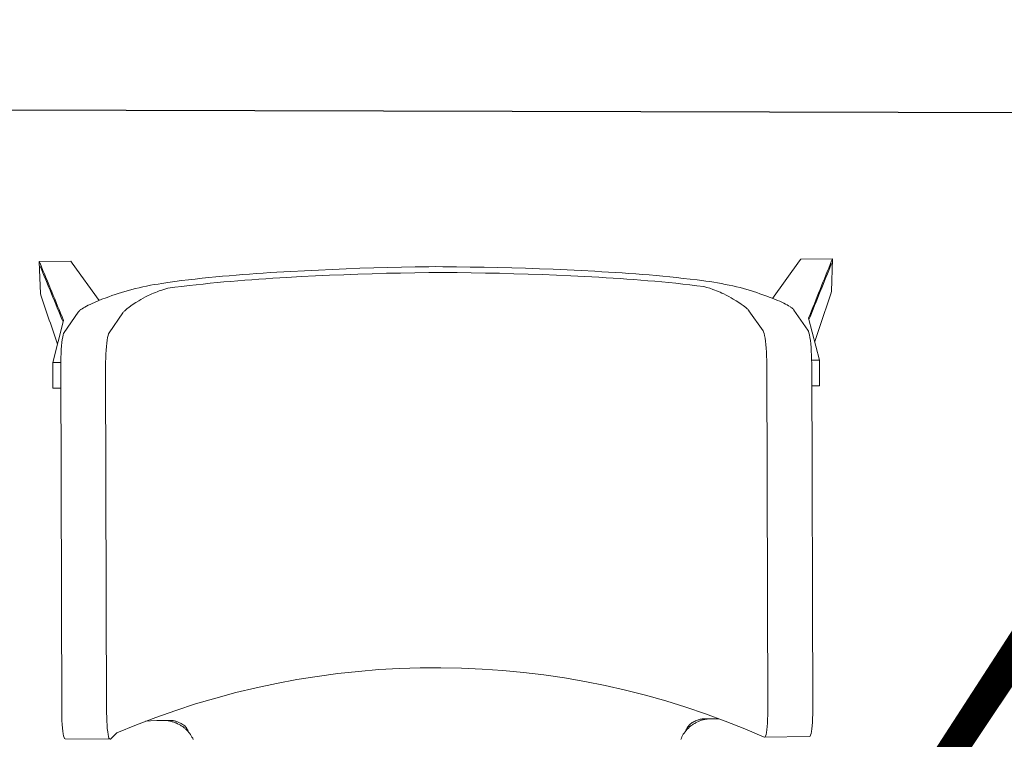
# Model space of a CAD drawing. Units: inches. Extents: x -466983 to 1020, y 324 to 318697.
# Tile 36 of 97: x 867.6 to 887.72, y 741.96 to 756.67. Entities that reach past the tile are written whole.
import ezdxf

# ---------------------------------------------------------------- set-up
doc = ezdxf.new("R2010")
doc.units = ezdxf.units.IN
doc.header["$MEASUREMENT"] = 0
for name, color, linetype, lineweight in [('A-ANNO-DIMS', 2, 'Continuous', 18), ('A-FLOR-PATT', 252, 'Continuous', 13), ('A-FURN', 8, 'Continuous', 18)]:
    doc.layers.add(name, color=color, linetype=linetype, lineweight=lineweight)
doc.layers.add('Office Desk', color=30, linetype='Continuous', true_color=0xeb7500)
doc.styles.get("Standard").update_dxf_attribs({"font": 'arial.ttf'})
doc.dimstyles.get("Standard").update_dxf_attribs({"dimtxt": 6, "dimasz": 4, "dimexe": 3, "dimexo": 3, "dimgap": 0.09, "dimtad": 0, "dimtih": 1, "dimtoh": 1, "dimdec": 1, "dimzin": 0, "dimdsep": 46, "dimlunit": 3, "dimtxsty": 'Standard', "dimcen": 0.09, "dimadec": 0, "dimazin": 0, "dimtfac": 1, "dimtdec": 1, "dimtofl": 0, "dimtmove": 0, "dimatfit": 3, "dimfxl": 1, "dimtolj": 1, "dimtzin": 0, "dimarcsym": 0})

# ---------------------------------------------------------------- blocks, each defined once
blk = doc.blocks.new('Offce Table')
at = {"layer": 'Office Desk'}
blk.add_line((2575.658, 950.355, -0.016), (2635.658, 950.194, -0.016), dxfattribs=at)
blk = doc.blocks.new('Office Chairs')
at = {"ltscale": 60}
for p, q in [((4347, 1436), (4348.4, 1437.9)), ((4382.1, 1438), (4348.4, 1437.9)), ((4382.1, 1438), (4381.1, 1403.3)), ((4382.1, 1438), (4381.3, 1436)), ((3537.6, 1435.4), (3571.3, 1435.6)), ((3537.6, 1435.4), (3538.4, 1433.4)), ((3537.6, 1435.4), (3538.8, 1400.8)), ((3572.7, 1433.6), (3571.3, 1435.6)), ((3601.5, 1393.8), (3572.7, 1433.6)), ((3820.1, 1425.5), (3834.9, 1426.2)), ((3834.9, 1426.2), (3849.6, 1426.9)), ((3849.6, 1426.9), (3864.3, 1427.5)), ((3864.3, 1427.5), (3879.1, 1428)), ((3879.1, 1428), (3893.8, 1428.4)), ((3893.8, 1428.4), (3908.6, 1428.8)), ((3908.6, 1428.8), (3923.3, 1429.2)), ((3923.3, 1429.2), (3937.9, 1429.5)), ((3937.9, 1429.5), (3952.6, 1429.7)), ((3952.6, 1429.7), (3959.9, 1429.8)), ((3967.2, 1429.7), (3959.9, 1429.8)), ((3981.9, 1429.6), (3967.2, 1429.7)), ((3996.5, 1429.4), (3981.9, 1429.6)), ((4011.3, 1429.2), (3996.5, 1429.4)), ((4026, 1428.8), (4011.3, 1429.2)), ((4040.8, 1428.5), (4026, 1428.8)), ((4055.5, 1428), (4040.8, 1428.5)), ((4070.3, 1427.5), (4055.5, 1428)), ((4085, 1427), (4070.3, 1427.5)), ((4099.8, 1426.3), (4085, 1427)), ((4114.5, 1425.6), (4099.8, 1426.3)), ((4318.5, 1396), (4347, 1436)), ((3689.2, 1414.9), (3696.5, 1415.7)), ((3696.5, 1415.7), (3703.8, 1416.6)), ((3703.8, 1416.6), (3711.1, 1417.4)), ((3711.1, 1417.4), (3718.3, 1418.1)), ((3718.3, 1418.1), (3725.5, 1418.8)), ((3725.5, 1418.8), (3732.8, 1419.5)), ((3732.8, 1419.5), (3740, 1420.1)), ((3740, 1420.1), (3747.2, 1420.7)), ((3747.2, 1420.7), (3754.4, 1421.3)), ((3749.1, 1414.7), (3756.5, 1415.3)), ((3754.4, 1421.3), (3761.6, 1421.9)), ((3756.5, 1415.3), (3763.9, 1415.9)), ((3761.6, 1421.9), (3768.9, 1422.4)), ((3763.9, 1415.9), (3771.4, 1416.4)), ((3768.9, 1422.4), (3776.1, 1422.9)), ((3771.4, 1416.4), (3778.8, 1416.9)), ((3776.1, 1422.9), (3783.4, 1423.4)), ((3778.8, 1416.9), (3786.3, 1417.4)), ((3783.4, 1423.4), (3790.7, 1423.8)), ((3786.3, 1417.4), (3793.8, 1417.9)), ((3790.7, 1423.8), (3805.4, 1424.7)), ((3793.8, 1417.9), (3801.3, 1418.3)), ((3801.3, 1418.3), (3816.4, 1419.2)), ((3805.4, 1424.7), (3820.1, 1425.5)), ((3816.4, 1419.2), (3831.6, 1419.9)), ((3831.6, 1419.9), (3846.7, 1420.6)), ((3846.7, 1420.6), (3861.8, 1421.2)), ((3861.8, 1421.2), (3877, 1421.8)), ((3877, 1421.8), (3892.1, 1422.3)), ((3892.1, 1422.3), (3907.2, 1422.7)), ((3907.2, 1422.7), (3922.4, 1423)), ((3922.4, 1423), (3937.4, 1423.3)), ((3937.4, 1423.3), (3952.4, 1423.6)), ((3952.4, 1423.6), (3959.9, 1423.6)), ((3967.5, 1423.6), (3959.9, 1423.6)), ((3982.5, 1423.5), (3967.5, 1423.6)), ((3997.5, 1423.3), (3982.5, 1423.5)), ((4012.7, 1423), (3997.5, 1423.3)), ((4027.8, 1422.7), (4012.7, 1423)), ((4042.9, 1422.3), (4027.8, 1422.7)), ((4058.1, 1421.8), (4042.9, 1422.3)), ((4073.2, 1421.3), (4058.1, 1421.8)), ((4088.3, 1420.7), (4073.2, 1421.3)), ((4103.5, 1420), (4088.3, 1420.7)), ((4118.6, 1419.3), (4103.5, 1420)), ((4129.2, 1424.9), (4114.5, 1425.6)), ((4126.1, 1418.9), (4118.6, 1419.3)), ((4133.6, 1418.5), (4126.1, 1418.9)), ((4136.5, 1424.4), (4129.2, 1424.9)), ((4141.1, 1418), (4133.6, 1418.5)), ((4143.8, 1424), (4136.5, 1424.4)), ((4148.6, 1417.6), (4141.1, 1418)), ((4151, 1423.5), (4143.8, 1424)), ((4156, 1417.1), (4148.6, 1417.6)), ((4158.3, 1423.1), (4151, 1423.5)), ((4163.4, 1416.6), (4156, 1417.1)), ((4165.5, 1422.6), (4158.3, 1423.1)), ((4170.8, 1416), (4163.4, 1416.6)), ((4172.7, 1422), (4165.5, 1422.6)), ((4178.2, 1415.4), (4170.8, 1416)), ((4179.9, 1421.5), (4172.7, 1422)), ((4185.6, 1414.8), (4178.2, 1415.4)), ((4187.1, 1420.9), (4179.9, 1421.5)), ((4194.4, 1420.2), (4187.1, 1420.9)), ((4201.6, 1419.6), (4194.4, 1420.2)), ((4208.9, 1418.9), (4201.6, 1419.6)), ((4216.1, 1418.1), (4208.9, 1418.9)), ((4223.4, 1417.3), (4216.1, 1418.1)), ((4230.7, 1416.5), (4223.4, 1417.3)), ((4238.1, 1415.6), (4230.7, 1416.5)), ((4245.4, 1414.7), (4238.1, 1415.6)), ((3632.5, 1404.4), (3636.2, 1405.4)), ((3636.2, 1405.4), (3640, 1406.4)), ((3640, 1406.4), (3643.9, 1407.3)), ((3643.9, 1407.3), (3647.9, 1408.2)), ((3647.9, 1408.2), (3651.9, 1409)), ((3651.9, 1409), (3656, 1409.9)), ((3656, 1409.9), (3660, 1410.6)), ((3660, 1410.6), (3664.2, 1411.3)), ((3664.2, 1411.3), (3668.3, 1412)), ((3665.3, 1403.9), (3668.3, 1404.9)), ((3668.3, 1412), (3672.5, 1412.6)), ((3668.3, 1404.9), (3671.4, 1405.9)), ((3671.4, 1405.9), (3674.6, 1406.8)), ((3672.5, 1412.6), (3674.5, 1412.9)), ((3674.5, 1412.9), (3681.9, 1413.9)), ((3674.6, 1406.8), (3682.1, 1407.8)), ((3681.9, 1413.9), (3689.2, 1414.9)), ((3682.1, 1407.8), (3689.6, 1408.8)), ((3689.6, 1408.8), (3697.1, 1409.7)), ((3697.1, 1409.7), (3704.6, 1410.5)), ((3704.6, 1410.5), (3712, 1411.3)), ((3712, 1411.3), (3719.5, 1412.1)), ((3719.5, 1412.1), (3726.9, 1412.8)), ((3726.9, 1412.8), (3734.3, 1413.5)), ((3734.3, 1413.5), (3741.7, 1414.1)), ((3741.7, 1414.1), (3749.1, 1414.7)), ((4193.1, 1414.2), (4185.6, 1414.8)), ((4200.5, 1413.5), (4193.1, 1414.2)), ((4207.9, 1412.8), (4200.5, 1413.5)), ((4215.4, 1412.1), (4207.9, 1412.8)), ((4222.9, 1411.3), (4215.4, 1412.1)), ((4230.4, 1410.4), (4222.9, 1411.3)), ((4237.9, 1409.5), (4230.4, 1410.4)), ((4245.4, 1408.5), (4237.9, 1409.5)), ((4247.5, 1414.4), (4245.4, 1414.7)), ((4248.6, 1407.6), (4245.4, 1408.5)), ((4251.6, 1413.8), (4247.5, 1414.4)), ((4251.7, 1406.7), (4248.6, 1407.6)), ((4255.8, 1413.1), (4251.6, 1413.8)), ((4254.7, 1405.6), (4251.7, 1406.7)), ((4256.8, 1404.9), (4254.7, 1405.6)), ((4259.9, 1412.4), (4255.8, 1413.1)), ((4258.8, 1404.2), (4256.8, 1404.9)), ((4264, 1411.7), (4259.9, 1412.4)), ((4268.1, 1410.9), (4264, 1411.7)), ((4272.1, 1410.1), (4268.1, 1410.9)), ((4276, 1409.2), (4272.1, 1410.1)), ((4279.9, 1408.3), (4276, 1409.2)), ((4283.8, 1407.4), (4279.9, 1408.3)), ((4287.5, 1406.4), (4283.8, 1407.4)), ((4291.2, 1405.4), (4287.5, 1406.4)), ((4294.8, 1404.3), (4291.2, 1405.4)), ((3539.6, 1398.4), (3538.8, 1400.8)), ((3600.3, 1393.3), (3604.4, 1395)), ((3604.4, 1395), (3608.8, 1396.7)), ((3608.8, 1396.7), (3611.8, 1397.8)), ((3611.8, 1397.8), (3615, 1398.9)), ((3615, 1398.9), (3618.3, 1400.1)), ((3618.3, 1400.1), (3621.7, 1401.2)), ((3621.7, 1401.2), (3625.2, 1402.3)), ((3625.2, 1402.3), (3628.8, 1403.4)), ((3628.8, 1403.4), (3632.5, 1404.4)), ((3643.5, 1393.4), (3645.9, 1394.8)), ((3645.9, 1394.8), (3648.4, 1396.2)), ((3648.4, 1396.2), (3650.9, 1397.6)), ((3650.9, 1397.6), (3653.6, 1399)), ((3653.6, 1399), (3655.5, 1399.9)), ((3655.5, 1399.9), (3657.4, 1400.7)), ((3657.4, 1400.7), (3659.3, 1401.5)), ((3659.3, 1401.5), (3661.3, 1402.3)), ((3661.3, 1402.3), (3663.2, 1403.1)), ((3663.2, 1403.1), (3665.3, 1403.9)), ((4260.7, 1403.4), (4258.8, 1404.2)), ((4262.7, 1402.6), (4260.7, 1403.4)), ((4264.5, 1401.7), (4262.7, 1402.6)), ((4266.4, 1400.9), (4264.5, 1401.7)), ((4269.1, 1399.5), (4266.4, 1400.9)), ((4271.7, 1398.1), (4269.1, 1399.5)), ((4274.2, 1396.7), (4271.7, 1398.1)), ((4276.6, 1395.3), (4274.2, 1396.7)), ((4279.6, 1393.5), (4276.6, 1395.3)), ((4298.3, 1403.2), (4294.8, 1404.3)), ((4301.7, 1402.1), (4298.3, 1403.2)), ((4305, 1401), (4301.7, 1402.1)), ((4308.2, 1399.9), (4305, 1401)), ((4311.3, 1398.8), (4308.2, 1399.9)), ((4315.7, 1397.1), (4311.3, 1398.8)), ((4319.8, 1395.5), (4315.7, 1397.1)), ((4323.6, 1393.9), (4319.8, 1395.5)), ((4380.3, 1401), (4381.1, 1403.3)), ((3581.4, 1383.7), (3581.9, 1384.1)), ((3581.9, 1384.1), (3582.5, 1384.5)), ((3582.5, 1384.5), (3583.2, 1385)), ((3583.2, 1385), (3584.6, 1385.9)), ((3584.6, 1385.9), (3586.2, 1386.8)), ((3586.2, 1386.8), (3587.9, 1387.7)), ((3587.9, 1387.7), (3589.8, 1388.7)), ((3589.8, 1388.7), (3591.9, 1389.6)), ((3591.9, 1389.6), (3594.1, 1390.7)), ((3594.1, 1390.7), (3596.4, 1391.7)), ((3596.4, 1391.7), (3600.3, 1393.3)), ((3629.4, 1383.6), (3630.1, 1384.2)), ((3630.1, 1384.2), (3631.4, 1385.3)), ((3631.4, 1385.3), (3632.9, 1386.4)), ((3632.9, 1386.4), (3635.2, 1388)), ((3635.2, 1388), (3637.7, 1389.7)), ((3637.7, 1389.7), (3640.5, 1391.5)), ((3640.5, 1391.5), (3643.5, 1393.4)), ((4282.4, 1391.7), (4279.6, 1393.5)), ((4284.9, 1390), (4282.4, 1391.7)), ((4287.2, 1388.4), (4284.9, 1390)), ((4288.7, 1387.3), (4287.2, 1388.4)), ((4290, 1386.2), (4288.7, 1387.3)), ((4290.8, 1385.6), (4290, 1386.2)), ((4291.5, 1385), (4290.8, 1385.6)), ((4292.1, 1384.4), (4291.5, 1385)), ((4292.6, 1383.8), (4292.1, 1384.4)), ((4326, 1392.9), (4323.6, 1393.9)), ((4328.2, 1391.9), (4326, 1392.9)), ((4330.3, 1390.9), (4328.2, 1391.9)), ((4332.2, 1390), (4330.3, 1390.9)), ((4333.9, 1389), (4332.2, 1390)), ((4335.5, 1388.1), (4333.9, 1389)), ((4337, 1387.3), (4335.5, 1388.1)), ((4337.6, 1386.8), (4337, 1387.3)), ((4338.2, 1386.4), (4337.6, 1386.8)), ((4338.8, 1386), (4338.2, 1386.4)), ((4339.3, 1385.6), (4338.8, 1386)), ((4339.7, 1385.2), (4339.3, 1385.6)), ((4340.2, 1384.8), (4339.7, 1385.2)), ((4340.5, 1384.4), (4340.2, 1384.8)), ((4340.9, 1384), (4340.5, 1384.4)), ((4341.2, 1383.6), (4340.9, 1384)), ((3564.2, 1359.8), (3579, 1381.3)), ((3579, 1381.3), (3579.3, 1381.7)), ((3579.3, 1381.7), (3579.6, 1382.1)), ((3579.6, 1382.1), (3580, 1382.5)), ((3580, 1382.5), (3580.4, 1382.9)), ((3580.4, 1382.9), (3580.9, 1383.3)), ((3580.9, 1383.3), (3581.4, 1383.7)), ((3612, 1359.2), (3626.8, 1380.7)), ((3626.8, 1380.7), (3627.1, 1381.2)), ((3627.1, 1381.2), (3627.6, 1381.8)), ((3627.6, 1381.8), (3628.1, 1382.3)), ((3628.1, 1382.3), (3628.7, 1382.9)), ((3628.7, 1382.9), (3629.4, 1383.6)), ((4293, 1383.2), (4292.6, 1383.8)), ((4293.3, 1382.7), (4293, 1383.2)), ((4308.3, 1361.3), (4293.3, 1382.7)), ((4356.1, 1362.2), (4341.2, 1383.6)), ((4368.5, 1330.2), (4356.7, 1375)), ((3552, 1327.7), (3563.5, 1372.6)), ((3562.1, 1352.1), (3562.6, 1354.8)), ((3562.6, 1354.8), (3563.1, 1357)), ((3563.1, 1357), (3563.6, 1358.7)), ((3563.6, 1358.7), (3564.2, 1359.8)), ((3610, 1351.4), (3610.4, 1354.2)), ((3610.4, 1354.2), (3610.9, 1356.4)), ((3610.9, 1356.4), (3611.5, 1358.1)), ((3611.5, 1358.1), (3612, 1359.2)), ((4308.3, 1361.3), (4308.9, 1360.2)), ((4308.9, 1360.2), (4309.4, 1358.5)), ((4309.4, 1358.5), (4309.9, 1356.3)), ((4309.9, 1356.3), (4310.4, 1353.6)), ((4310.4, 1353.6), (4310.9, 1350.4)), ((4356.1, 1362.2), (4356.7, 1361.1)), ((4356.7, 1361.1), (4357.2, 1359.4)), ((4357.2, 1359.4), (4357.8, 1357.2)), ((4357.8, 1357.2), (4358.2, 1354.5)), ((4358.2, 1354.5), (4358.7, 1351.3)), ((3561, 1341.4), (3561.3, 1345.3)), ((3561.3, 1345.3), (3561.7, 1348.9)), ((3561.7, 1348.9), (3562.1, 1352.1)), ((3608.8, 1340.8), (3609.2, 1344.7)), ((3609.2, 1344.7), (3609.5, 1348.3)), ((3609.5, 1348.3), (3610, 1351.4)), ((4310.9, 1350.4), (4311.2, 1346.8)), ((4311.2, 1346.8), (4311.6, 1342.9)), ((4311.6, 1342.9), (4311.9, 1338.8)), ((4358.7, 1351.3), (4359.1, 1347.7)), ((4359.1, 1347.7), (4359.4, 1343.8)), ((4359.4, 1343.8), (4359.7, 1339.7)), ((3560.5, 1328.5), (3560.6, 1333)), ((3560.6, 1333), (3560.8, 1337.3)), ((3560.8, 1337.3), (3561, 1341.4)), ((3608.3, 1327.9), (3608.4, 1332.3)), ((3608.4, 1332.3), (3608.6, 1336.6)), ((3608.6, 1336.6), (3608.8, 1340.8)), ((4311.9, 1338.8), (4312.1, 1334.5)), ((4312.1, 1334.5), (4312.2, 1330.1)), ((4359.7, 1339.7), (4359.9, 1335.4)), ((4359.9, 1335.4), (4360, 1331)), ((3552, 1327.7), (3555.2, 1327.7)), ((3552, 1325.1), (3552, 1327.7)), ((3552.2, 1300.3), (3552, 1325.1)), ((3555.2, 1327.7), (3560.5, 1327.6)), ((3560.5, 1324.1), (3560.5, 1328.5)), ((3561.6, 955.2), (3560.5, 1324.1)), ((3608.3, 1323.5), (3608.3, 1327.9)), ((3609.4, 954.5), (3608.3, 1323.5)), ((4312.2, 1330.1), (4312.2, 1325.6)), ((4313.4, 956.7), (4312.2, 1325.6)), ((4360, 1331), (4360.1, 1326.6)), ((4365.3, 1330.1), (4360, 1330.1)), ((4361.2, 957.6), (4360.1, 1326.6)), ((4368.5, 1330.2), (4365.3, 1330.1)), ((4368.5, 1327.6), (4368.5, 1330.2)), ((4368.5, 1302.8), (4368.5, 1327.6)), ((3552.2, 1300.3), (3560.5, 1300.3)), ((4368.5, 1302.8), (4360.1, 1302.7)), ((3561.6, 950.6), (3561.6, 955.2)), ((3609.5, 950), (3609.4, 954.5)), ((4313.4, 956.7), (4313.3, 952.1)), ((4361.2, 957.6), (4361.2, 953.1)), ((3561.8, 946.3), (3561.6, 950.6)), ((3562, 942.2), (3561.8, 946.3)), ((3609.6, 945.6), (3609.5, 950)), ((3609.8, 941.5), (3609.6, 945.6)), ((3650.6, 945.6), (3656.2, 946)), ((3656.2, 946), (3662.8, 946.3)), ((3662.8, 946.3), (3669.7, 946.5)), ((3670.6, 946.5), (3669.7, 946.5)), ((3671.4, 946.5), (3670.6, 946.5)), ((3672.3, 946.5), (3671.4, 946.5)), ((3673.1, 946.4), (3672.3, 946.5)), ((3674, 946.3), (3673.1, 946.4)), ((3674.8, 946.2), (3674, 946.3)), ((3675.7, 946), (3674.8, 946.2)), ((3676.5, 945.9), (3675.7, 946)), ((3677.3, 946.6), (3675.9, 946.6)), ((3677.4, 945.7), (3676.5, 945.9)), ((3678.8, 946.4), (3677.3, 946.6)), ((3678.2, 945.5), (3677.4, 945.7)), ((3679.1, 945.2), (3678.2, 945.5)), ((3679.5, 946.4), (3678.8, 946.4)), ((3679.9, 945), (3679.1, 945.2)), ((3680.2, 946.3), (3679.5, 946.4)), ((3680.8, 944.7), (3679.9, 945)), ((3680.9, 946.1), (3680.2, 946.3)), ((3681.6, 944.4), (3680.8, 944.7)), ((3681.6, 946), (3680.9, 946.1)), ((3682.2, 945.8), (3681.6, 946)), ((3682.5, 944.1), (3681.6, 944.4)), ((3682.9, 945.6), (3682.2, 945.8)), ((3683.3, 943.8), (3682.5, 944.1)), ((3683.6, 945.4), (3682.9, 945.6)), ((3684.9, 943), (3683.3, 943.8)), ((3686.9, 944.1), (3686.3, 944.3)), ((3687.9, 943.7), (3686.9, 944.1)), ((3688.9, 943.2), (3687.9, 943.7)), ((4231.1, 942.9), (4232, 943.6)), ((4232, 943.6), (4232.9, 944.3)), ((4232.9, 944.3), (4233.9, 944.8)), ((4233.9, 944.8), (4234.9, 945.3)), ((4234.9, 945.3), (4235.9, 945.8)), ((4235.5, 943.4), (4236.2, 943.9)), ((4235.9, 945.8), (4236.4, 946)), ((4236.2, 943.9), (4237.8, 944.7)), ((4237.8, 944.7), (4239.5, 945.4)), ((4239.2, 947.1), (4239.9, 947.3)), ((4239.5, 945.4), (4240.3, 945.8)), ((4239.9, 947.3), (4240.5, 947.5)), ((4240.3, 945.8), (4241.1, 946.1)), ((4240.5, 947.5), (4241.2, 947.7)), ((4241.1, 946.1), (4242, 946.4)), ((4241.2, 947.7), (4241.9, 947.8)), ((4241.9, 947.8), (4242.6, 948)), ((4242, 946.4), (4242.8, 946.7)), ((4242.6, 948), (4243.3, 948.1)), ((4242.8, 946.7), (4243.7, 947)), ((4243.3, 948.1), (4244, 948.2)), ((4243.7, 947), (4244.5, 947.2)), ((4244, 948.2), (4245.4, 948.3)), ((4244.5, 947.2), (4245.4, 947.4)), ((4245.4, 948.3), (4246.9, 948.3)), ((4245.4, 947.4), (4246.2, 947.6)), ((4246.2, 947.6), (4247.1, 947.8)), ((4247.1, 947.8), (4248, 947.9)), ((4248, 947.9), (4248.8, 948)), ((4248.8, 948), (4249.7, 948.1)), ((4249.7, 948.1), (4250.5, 948.2)), ((4250.5, 948.2), (4251.4, 948.3)), ((4251.4, 948.3), (4252.2, 948.3)), ((4252.2, 948.3), (4253.1, 948.3)), ((4253.1, 948.3), (4260, 948.1)), ((4260, 948.1), (4262.3, 948)), ((4313, 943.7), (4312.7, 939.9)), ((4313.2, 947.8), (4313, 943.7)), ((4313.3, 952.1), (4313.2, 947.8)), ((4360.9, 944.6), (4360.6, 940.9)), ((4361, 948.7), (4360.9, 944.6)), ((4361.2, 953.1), (4361, 948.7)), ((3562.3, 938.4), (3562, 942.2)), ((3562.6, 935.1), (3562.3, 938.4)), ((3563.1, 932.3), (3562.6, 935.1)), ((3610.1, 937.8), (3609.8, 941.5)), ((3610.5, 934.5), (3610.1, 937.8)), ((3610.9, 931.7), (3610.5, 934.5)), ((3620.2, 933.3), (3613.5, 926.7)), ((3686.6, 942.2), (3684.9, 943)), ((3687.3, 941.8), (3686.6, 942.2)), ((3688.1, 941.3), (3687.3, 941.8)), ((3688.9, 940.8), (3688.1, 941.3)), ((3689.9, 942.6), (3688.9, 943.2)), ((3689.6, 940.4), (3688.9, 940.8)), ((3690.4, 939.9), (3689.6, 940.4)), ((3690.8, 942), (3689.9, 942.6)), ((3691.1, 939.3), (3690.4, 939.9)), ((3691.7, 941.3), (3690.8, 942)), ((3691.8, 938.8), (3691.1, 939.3)), ((3692.5, 940.6), (3691.7, 941.3)), ((3692.5, 938.3), (3691.8, 938.8)), ((3693.3, 939.8), (3692.5, 940.6)), ((3693.1, 937.7), (3692.5, 938.3)), ((3693.8, 937.1), (3693.1, 937.7)), ((3694, 938.9), (3693.3, 939.8)), ((3694.4, 936.5), (3693.8, 937.1)), ((3694.7, 938), (3694, 938.9)), ((3695, 935.9), (3694.4, 936.5)), ((3695.3, 937), (3694.7, 938)), ((3695.6, 935.3), (3695, 935.9)), ((3695.8, 936.1), (3695.3, 937)), ((3696.2, 934.7), (3695.6, 935.3)), ((3696.3, 935.1), (3695.8, 936.1)), ((3696.7, 934), (3696.2, 934.7)), ((3696.7, 934), (3696.3, 935.1)), ((3696.7, 934), (3697.7, 932.8)), ((4224.2, 933.1), (4223.4, 931.8)), ((4225.2, 934.4), (4224.2, 933.1)), ((4226.1, 935.6), (4225.2, 934.4)), ((4226.1, 935.6), (4226.6, 936.7)), ((4226.1, 935.6), (4226.7, 936.3)), ((4226.6, 936.7), (4227, 937.7)), ((4226.7, 936.3), (4227.2, 936.9)), ((4227, 937.7), (4227.6, 938.7)), ((4227.2, 936.9), (4227.8, 937.5)), ((4227.6, 938.7), (4228.2, 939.6)), ((4227.8, 937.5), (4228.4, 938.1)), ((4228.2, 939.6), (4228.8, 940.5)), ((4228.4, 938.1), (4229.1, 938.7)), ((4228.8, 940.5), (4229.5, 941.4)), ((4229.1, 938.7), (4229.7, 939.3)), ((4229.5, 941.4), (4230.3, 942.2)), ((4229.7, 939.3), (4230.4, 939.9)), ((4230.3, 942.2), (4231.1, 942.9)), ((4230.4, 939.9), (4231.1, 940.4)), ((4231.1, 940.4), (4231.7, 941)), ((4231.7, 941), (4232.5, 941.5)), ((4232.5, 941.5), (4233.2, 942)), ((4233.2, 942), (4233.9, 942.5)), ((4233.9, 942.5), (4234.7, 943)), ((4234.7, 943), (4235.5, 943.4)), ((4312, 933.8), (4311.5, 931.6)), ((4312.4, 936.6), (4312, 933.8)), ((4312.7, 939.9), (4312.4, 936.6)), ((4359.8, 934.7), (4359.4, 932.5)), ((4360.2, 937.6), (4359.8, 934.7)), ((4360.6, 940.9), (4360.2, 937.6)), ((3563.5, 930.1), (3563.1, 932.3)), ((3564.1, 928.4), (3563.5, 930.1)), ((3564.6, 927.4), (3564.1, 928.4)), ((3565.2, 927.1), (3564.6, 927.4)), ((3613, 926.5), (3565.2, 927.1)), ((3611.4, 929.4), (3610.9, 931.7)), ((3611.9, 927.8), (3611.4, 929.4)), ((3612.5, 926.8), (3611.9, 927.8)), ((3613, 926.5), (3612.5, 926.8)), ((3613.1, 926.5), (3613, 926.5)), ((3613.2, 926.5), (3613.1, 926.5)), ((3613.1, 926.5), (3613.1, 926.5)), ((3613.3, 926.5), (3613.2, 926.5)), ((3613.4, 926.6), (3613.3, 926.5)), ((3613.3, 926.5), (3613.3, 926.5)), ((3613.5, 926.7), (3613.4, 926.6)), ((3613.4, 926.6), (3613.4, 926.6)), ((3613.5, 926.7), (3613.5, 926.7)), ((3697.7, 932.8), (3698.6, 931.5)), ((3698.6, 931.5), (3699.5, 930.2)), ((3699.5, 930.2), (3700.2, 928.8)), ((3700.2, 928.8), (3701, 927.5)), ((3701, 927.5), (3701.6, 926.1)), ((4221.3, 927.7), (4220.7, 926.3)), ((4221.9, 929.1), (4221.3, 927.7)), ((4222.6, 930.4), (4221.9, 929.1)), ((4223.4, 931.8), (4222.6, 930.4)), ((4309.5, 928.7), (4309.4, 928.8)), ((4309.4, 928.8), (4309.4, 928.8)), ((4309.6, 928.7), (4309.5, 928.7)), ((4309.6, 928.6), (4309.6, 928.7)), ((4309.7, 928.6), (4309.6, 928.6)), ((4309.8, 928.6), (4309.7, 928.6)), ((4309.7, 928.6), (4309.7, 928.6)), ((4309.9, 928.6), (4309.8, 928.6)), ((4309.8, 928.6), (4309.8, 928.6)), ((4357.7, 929.5), (4309.9, 928.6)), ((4310.5, 928.9), (4309.9, 928.6)), ((4311, 929.9), (4310.5, 928.9)), ((4311.5, 931.6), (4311, 929.9)), ((4358.3, 929.8), (4357.7, 929.5)), ((4358.8, 930.8), (4358.3, 929.8)), ((4359.4, 932.5), (4358.8, 930.8))]:
    blk.add_line(p, q, dxfattribs=at)
for centre, radius, start, end in [((-144223, -59409.2), 159797.6, 22.356435, 22.380032), ((-143343.5, -59049.8), 158846.4, 22.356749, 22.380057), ((152380.7, -58271.4), 159589.4, 158.029376, 158.052995), ((151495, -57916.8), 158634.4, 158.029363, 158.052681), ((-167010.2, -56961.5), 180258.5, 18.873132, 18.89027), ((175076.3, -55674.8), 179985.4, 161.511556, 161.528687), ((3677.2, 568.1), 378.5, 90.1872, 91.127), ((3677.8, 926.7), 19.6, 64.1372, 72.7729), ((4245.1, 928.4), 19.6, 107.5751, 116.2106), ((4247.9, 569.8), 378.5, 89.2211, 90.1609)]:
    blk.add_arc(centre, radius, start, end, dxfattribs=at)
blk.add_arc((3959.7, 138.9), 863.8, 66.1195, 113.1374)
blk = doc.blocks.new('Office Desk With Chairs')
blk.add_blockref('Offce Table', (-526.404, 94.584))
at = {"xscale": 0.0191941550942558, "yscale": 0.0191941550942558, "zscale": 0.0191941550942558}
blk.add_blockref('Office Chairs', (2012.509, 1014.21), dxfattribs=at)
blk = doc.blocks.new('*D91')
at = {"layer": 'A-ANNO-DIMS', "color": 0, "lineweight": -2, "transparency": 16777216}
for p, q in [((938.253, 802.547), (920.07, 802.547)), ((923.07, 798.547), (923.07, 745.132)), ((923.07, 685.328), (923.07, 738.743)), ((938.253, 681.328), (920.07, 681.328))]:
    blk.add_line(p, q, dxfattribs=at)
at = {"layer": 'A-ANNO-DIMS', "color": 0, "transparency": 16777216}
for points in [[(922.404, 798.547), (923.737, 798.547), (923.07, 802.547)], [(922.404, 685.328), (923.737, 685.328), (923.07, 681.328)]]:
    blk.add_solid(points, dxfattribs=at)
at = {"layer": 'Defpoints', "color": 0, "transparency": 16777216}
for p in [(941.253, 802.547), (923.07, 681.328), (941.253, 681.328)]:
    blk.add_point(p, dxfattribs=at)
at = {"layer": 'A-ANNO-DIMS', "color": 0, "transparency": 16777216, "insert": (923.07, 741.937), "char_height": 6, "attachment_point": 5}
blk.add_mtext('\\A1;4-SEATER SOFA 121', dxfattribs=at)

msp = doc.modelspace()

# ---------------------------------------------------------------- hatches: boundary and pattern name
at = {"layer": 'A-FLOR-PATT', "transparency": 33554572}
h = msp.add_hatch(dxfattribs=at)
h.set_pattern_fill('ANSI37', color=256, scale=30)
h.set_pattern_definition([(45, (-1212.4137, -290.035), (-2.6516504, 2.6516504), []), (135, (-1212.4137, -290.035), (-2.6516504, -2.6516504), [])])
h.paths.add_polyline_path([(901.806, 1075.938), (900.614, 1075.938), (900.614, 1065.386), (899.391, 1065.386), (898.091, 1065.386), (892.836, 1058.71, -0.258377), (892.188, 1058.351), (879.985, 1058.351, -0.20177), (879.438, 1058.581), (874.081, 1065.386), (872.781, 1065.386), (871.558, 1065.386), (871.558, 1075.938), (813.806, 1075.938), (813.806, 1044.792), (832.395, 1044.792, -0.394795), (848.66, 1028.536), (848.66, 1009.938), (901.806, 1009.938), (901.806, 1015.938), (901.306, 1015.938), (871.306, 1015.938), (871.306, 1017.25), (871.334, 1017.25, -0.401453), (901.306, 1045.938), (901.806, 1045.938)])
edge = h.paths.add_edge_path(flags=16)
edge.add_line((847.773, 1068.949), (847.773, 1073.709))
edge.add_arc((849.227, 1073.709), 1.454, 90, 180, ccw=False)
edge.add_line((849.227, 1075.163), (864.492, 1075.163))
edge.add_arc((864.492, 1073.709), 1.454, 0, 90, ccw=False)
edge.add_line((865.946, 1073.709), (865.946, 1069.004))
edge.add_arc((832.645, 1068.976), 33.301, -20.6123, 0.0472, ccw=False)
edge.add_ellipse((856.859, 1058.48), major_axis=(0, 10.213), ratio=0.685919, start_angle=100.0088, end_angle=259.9912, ccw=False)
edge.add_arc((881.074, 1068.976), 33.301, 180.0472, 200.6123, ccw=False)
h.paths.add_polyline_path([(853.146, 1066.482), (853.146, 1066.453), (853.146, 1066.453, 0.433107), (852.917, 1066.685), (852.917, 1066.453), (853.146, 1066.453), (853.146, 1066.482), (853.088, 1066.612, 0.697939), (852.7, 1066.453), (852.7, 1066.453), (852.7, 1066.482), (852.917, 1067.001), (852.917, 1066.685, -0.396254)], flags=0)
h.paths.add_polyline_path([(861.019, 1066.482), (861.019, 1066.453), (861.019, 1066.453, 0.416404), (860.802, 1066.685), (860.802, 1066.453), (861.019, 1066.453), (861.019, 1066.482), (860.967, 1066.605, 0.713344), (860.573, 1066.453), (860.573, 1066.453), (860.573, 1066.482), (860.802, 1067.001), (860.802, 1066.685, -0.379973)], flags=0)
edge = h.paths.add_edge_path(flags=0)
edge.add_spline(control_points=[(861.13, 1065.785), (861.466, 1065.248), (861.613, 1065.016), (861.983, 1064.374), (862.192, 1063.944), (862.561, 1063.039), (862.721, 1062.563), (862.987, 1061.578), (863.092, 1061.069), (863.245, 1060.031), (863.293, 1059.503), (863.329, 1058.441), (863.318, 1057.908), (863.237, 1056.852), (863.166, 1056.329), (862.97, 1055.308), (862.843, 1054.81), (862.537, 1053.852), (862.357, 1053.393), (861.951, 1052.525), (861.725, 1052.117), (861.233, 1051.362), (860.967, 1051.016), (860.405, 1050.395), (860.108, 1050.12), (859.494, 1049.646), (859.176, 1049.448), (858.528, 1049.13), (858.197, 1049.011), (857.531, 1048.852), (857.196, 1048.812), (856.525, 1048.812), (856.189, 1048.852), (855.524, 1049.01), (855.193, 1049.129), (854.545, 1049.447), (854.227, 1049.645), (853.612, 1050.118), (853.316, 1050.393), (852.753, 1051.014), (852.487, 1051.36), (851.995, 1052.114), (851.769, 1052.523), (851.363, 1053.39), (851.183, 1053.85), (850.877, 1054.807), (850.75, 1055.305), (850.553, 1056.326), (850.483, 1056.849), (850.401, 1057.905), (850.39, 1058.438), (850.426, 1059.5), (850.473, 1060.028), (850.626, 1061.066), (850.732, 1061.575), (850.997, 1062.561), (851.157, 1063.036), (851.525, 1063.942), (851.734, 1064.371), (852.106, 1065.016), (852.254, 1065.25), (852.608, 1065.733)], knot_values=[3.915332, 3.915332, 3.915332, 3.915332, 4.013468, 4.013468, 4.175532, 4.175532, 4.337596, 4.337596, 4.49966, 4.49966, 4.661724, 4.661724, 4.823788, 4.823788, 4.985852, 4.985852, 5.147916, 5.147916, 5.30998, 5.30998, 5.472044, 5.472044, 5.634109, 5.634109, 5.796173, 5.796173, 5.958237, 5.958237, 6.120301, 6.120301, 6.282365, 6.282365, 6.444429, 6.444429, 6.606493, 6.606493, 6.768557, 6.768557, 6.930621, 6.930621, 7.092685, 7.092685, 7.254749, 7.254749, 7.416813, 7.416813, 7.578878, 7.578878, 7.740942, 7.740942, 7.903006, 7.903006, 8.06507, 8.06507, 8.227134, 8.227134, 8.389198, 8.389198, 8.551262, 8.551262, 8.65037, 8.65037, 8.65037, 8.65037], degree=3, periodic=0)
edge.add_line((852.642, 1065.785), (861.13, 1065.785))
edge = h.paths.add_edge_path(flags=0)
edge.add_ellipse((856.85, 1057.743), major_axis=(0, 7.792), ratio=0.687861, start_angle=0, end_angle=360)
h.paths.add_polyline_path([(848.863, 1069.389), (848.863, 1073.96, -0.414214), (849.954, 1075.051), (863.765, 1075.051, -0.414214), (864.856, 1073.96), (864.856, 1069.389, -0.388936), (864.524, 1069.027, -0.043561), (849.195, 1069.027, -0.388936)], flags=0)
h.paths.add_polyline_path([(853.101, 1068.112, -1), (852.677, 1068.112, -1)], flags=0)
edge = h.paths.add_edge_path(flags=0)
edge.add_ellipse((856.859, 1057.338), major_axis=(0, 2.207), ratio=0.657164, start_angle=0, end_angle=360)
h.paths.add_polyline_path([(861.041, 1068.112, -1), (860.618, 1068.112, -1)], flags=0)
edge = h.paths.add_edge_path()
edge.add_line((573.954, 1057.341), (573.954, 1075.938))
edge.add_line((573.954, 1075.938), (558.731, 1075.938))
edge.add_line((558.731, 1075.938), (558.731, 1065.386))
edge.add_line((558.731, 1065.386), (557.507, 1065.386))
edge.add_line((557.507, 1065.386), (556.207, 1065.386))
edge.add_line((556.207, 1065.386), (550.952, 1058.71))
edge.add_arc((550.304, 1059.116), 0.765, 270, 327.9483, ccw=False)
edge.add_line((550.304, 1058.351), (538.101, 1058.351))
edge.add_arc((538.101, 1059.116), 0.765, 224.3704, 270, ccw=False)
edge.add_line((537.555, 1058.581), (532.198, 1065.386))
edge.add_line((532.198, 1065.386), (530.898, 1065.386))
edge.add_line((530.898, 1065.386), (529.674, 1065.386))
edge.add_line((529.674, 1065.386), (529.674, 1075.938))
edge.add_line((529.674, 1075.938), (520.806, 1075.938))
edge.add_line((520.806, 1075.938), (520.806, 1045.938))
edge.add_line((520.806, 1045.938), (521.306, 1045.938))
edge.add_arc((521.306, 1015.938), 30, 2.5075, 90, ccw=False)
edge.add_line((551.277, 1017.25), (551.306, 1017.25))
edge.add_line((551.306, 1017.25), (551.306, 1015.938))
edge.add_line((551.306, 1015.938), (520.806, 1015.938))
edge.add_line((520.806, 1015.938), (520.806, 1009.938))
edge.add_line((520.806, 1009.938), (559.191, 1010.402))
edge.add_arc((559.191, 1011.856), 1.454, 180, 270, ccw=False)
edge.add_line((557.737, 1011.856), (557.737, 1016.561))
edge.add_arc((591.039, 1016.589), 33.301, 159.3877, 180.0472, ccw=False)
edge.add_ellipse((566.824, 1027.085), major_axis=(0, 10.213), ratio=0.685919, start_angle=280.0088, end_angle=439.9912, ccw=False)
edge.add_arc((542.609, 1016.589), 33.301, 0.0472, 20.6123, ccw=False)
edge.add_line((575.91, 1016.616), (575.91, 1011.856))
edge.add_arc((574.456, 1011.856), 1.454, -90, 0, ccw=False)
edge.add_line((574.456, 1010.402), (608.806, 1009.938))
edge.add_line((608.806, 1009.938), (608.806, 1041.086))
edge.add_line((608.806, 1041.086), (590.218, 1041.086))
edge.add_arc((590.775, 1057.907), 16.831, 181.9277, 268.1032, ccw=False)
edge = h.paths.add_edge_path()
edge.add_ellipse((494.244, 583.62), major_axis=(0, 10.213), ratio=0.685919, start_angle=280.0088, end_angle=439.9912, ccw=False)
edge.add_arc((470.03, 573.124), 33.301, 0.0472, 20.6123, ccw=False)
edge.add_line((503.331, 573.152), (503.331, 568.392))
edge.add_arc((501.877, 568.392), 1.454, -90, 0, ccw=False)
edge.add_line((501.877, 566.938), (539.806, 566.938))
edge.add_line((539.806, 566.938), (539.806, 572.938))
edge.add_line((539.806, 572.938), (539.306, 572.938))
edge.add_line((539.306, 572.938), (509.306, 572.938))
edge.add_line((509.306, 572.938), (509.306, 574.25))
edge.add_line((509.306, 574.25), (509.334, 574.25))
edge.add_arc((539.306, 572.938), 30, 90, 177.4925, ccw=False)
edge.add_line((539.306, 602.938), (539.806, 602.938))
edge.add_line((539.806, 602.938), (539.806, 626.938))
edge.add_line((539.806, 626.938), (531.772, 626.938))
edge.add_line((531.772, 626.938), (531.772, 616.386))
edge.add_line((531.772, 616.386), (530.548, 616.386))
edge.add_line((530.548, 616.386), (529.249, 616.386))
edge.add_line((529.249, 616.386), (523.711, 609.351))
edge.add_line((523.711, 609.351), (510.777, 609.351))
edge.add_line((510.777, 609.351), (505.239, 616.386))
edge.add_line((505.239, 616.386), (503.939, 616.386))
edge.add_line((503.939, 616.386), (502.715, 616.386))
edge.add_line((502.715, 616.386), (502.715, 626.938))
edge.add_line((502.715, 626.938), (481.698, 626.938))
edge.add_line((481.698, 626.938), (481.698, 610.995))
edge.add_arc((467.27, 611.473), 14.436, 271.9277, 358.1032, ccw=False)
edge.add_line((467.756, 597.045), (451.806, 597.045))
edge.add_line((451.806, 597.045), (451.806, 584.404))
edge.add_line((451.806, 584.404), (451.806, 566.938))
edge.add_line((451.806, 566.938), (486.612, 566.938))
edge.add_arc((486.612, 568.392), 1.454, 180, 270, ccw=False)
edge.add_line((485.158, 568.392), (485.158, 573.097))
edge.add_arc((518.459, 573.124), 33.301, 159.3877, 180.0472, ccw=False)
h.paths.add_polyline_path([(836.261, 1020.733), (879.89, 1020.733), (879.89, 1039.39), (836.261, 1039.39)], flags=25)
h.paths.add_polyline_path([(549.985, 1036.749), (593.614, 1036.749), (593.614, 1055.407), (549.985, 1055.407)], flags=24)
h.paths.add_polyline_path([(475.123, 595.596), (518.752, 595.596), (518.752, 614.253), (475.123, 614.253)], flags=24)

# ---------------------------------------------------------------- block references
at = {"layer": 'A-FURN'}
msp.add_blockref('Office Desk With Chairs', (-1212.414, -290.035), dxfattribs=at)

# ---------------------------------------------------------------- dimensions: what is measured, and where the dimension line sits
at = {"layer": 'A-ANNO-DIMS'}
dim = msp.add_linear_dim(base=(923.07, 681.328), p1=(941.253, 802.547), p2=(941.253, 681.328), angle=270, text='4-SEATER SOFA <>', dimstyle='Standard', override={"dimdec": 0, "dimlfac": 1, "dimrnd": 0, "dimzin": 0, "dimdsep": 46, "dimlunit": 2}, dxfattribs=at)
dim.commit()
dim.dimension.update_dxf_attribs({"geometry": '*D91', "text_midpoint": (923.07, 741.937)})

doc.saveas('drawing.dxf')
